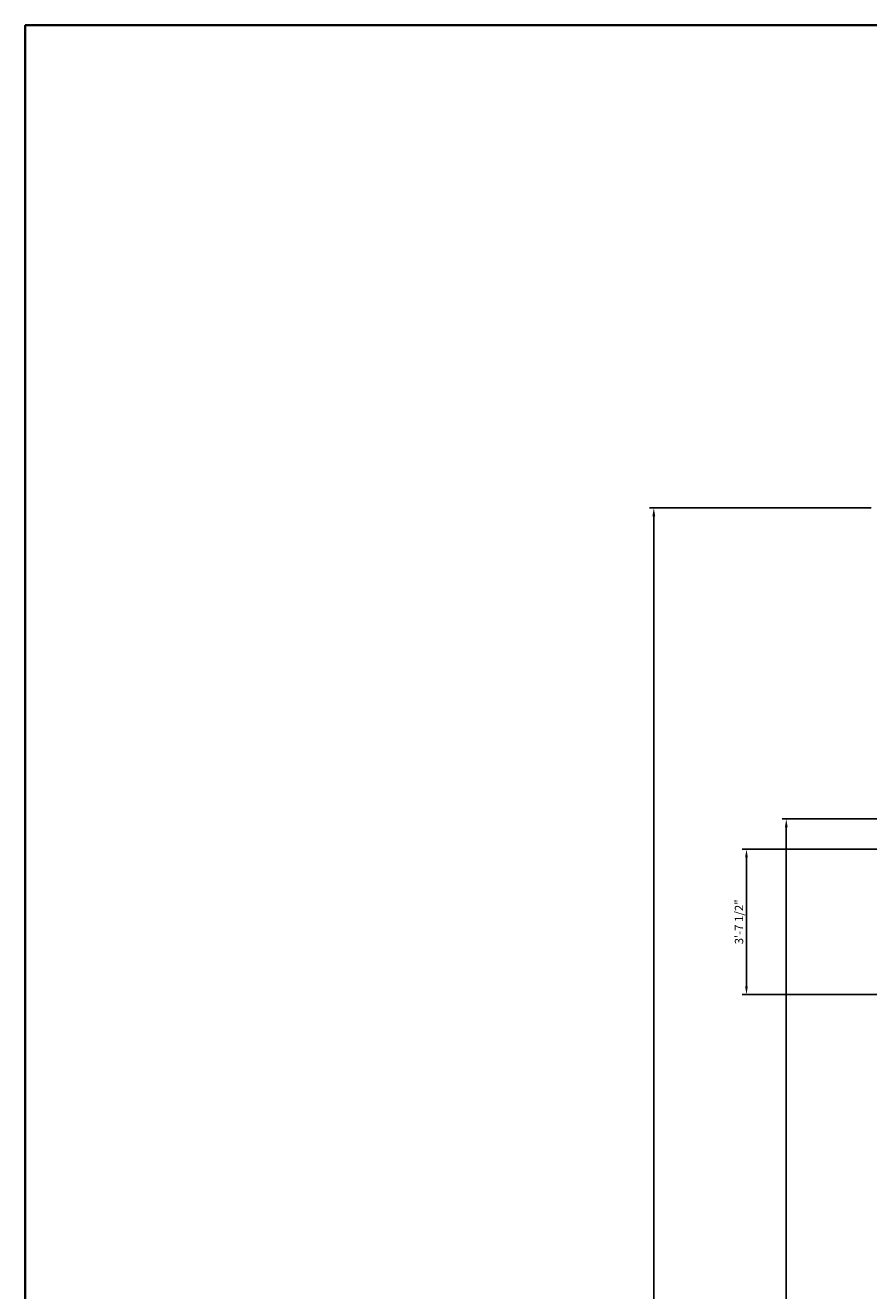
# Model space of a CAD drawing. Units: inches. Extents: x 6038 to 7543, y 3772 to 5131.
# Tile 7 of 14: x 6038 to 6290, y 4753 to 5131. Entities that reach past the tile are written whole.
import ezdxf

# ---------------------------------------------------------------- set-up
doc = ezdxf.new("R2010")
doc.units = ezdxf.units.IN
doc.layers.add('A-ANNO-DIMS', color=4, linetype='Continuous', lineweight=18)
doc.layers.add('A-ANNO-TTLB', color=1, linetype='Continuous', lineweight=35)
doc.styles.get("Standard").update_dxf_attribs({"font": 'arial.ttf'})
doc.dimstyles.new('ISO-25', dxfattribs={"dimtxt": 2.5, "dimasz": 2.5, "dimexe": 1.25, "dimexo": 0.625, "dimtad": 1, "dimdec": 0, "dimlunit": 3, "dimtxsty": 'Standard', "dimcen": 2.5, "dimadec": 0, "dimazin": 0, "dimtfac": 1, "dimtdec": 0, "dimtmove": 0, "dimatfit": 3, "dimfxl": 1, "dimarcsym": 0})

# ---------------------------------------------------------------- blocks, each defined once
blk = doc.blocks.new('*D15')
at = {"layer": 'A-ANNO-DIMS', "color": 0, "lineweight": -2, "transparency": 16777216}
for p, q in [((6320.79, 4893.62), (6264.12, 4893.62)), ((6265.37, 4891.12), (6265.37, 4551.12)), ((6320.79, 4548.62), (6264.12, 4548.62))]:
    blk.add_line(p, q, dxfattribs=at)
at = {"layer": 'A-ANNO-DIMS', "color": 0, "transparency": 16777216}
for points in [[(6264.96, 4891.12), (6265.79, 4891.12), (6265.37, 4893.62)], [(6264.96, 4551.12), (6265.79, 4551.12), (6265.37, 4548.62)]]:
    blk.add_solid(points, dxfattribs=at)
at = {"layer": 'Defpoints', "color": 0, "transparency": 16777216}
for p in [(6321.42, 4893.62), (6265.37, 4548.62), (6321.42, 4548.62)]:
    blk.add_point(p, dxfattribs=at)
at = {"layer": 'A-ANNO-DIMS', "color": 0, "transparency": 16777216, "insert": (6257.09, 4721.12), "char_height": 2.5, "attachment_point": 5, "rotation": 90}
blk.add_mtext('{\\H6x;28\'-9"}', dxfattribs=at)
blk = doc.blocks.new('*D17')
at = {"layer": 'A-ANNO-DIMS', "color": 0, "lineweight": -2, "transparency": 16777216}
for p, q in [((6290.79, 4986.62), (6224.51, 4986.62)), ((6225.76, 4984.12), (6225.76, 4365.12)), ((6290.79, 4362.62), (6224.51, 4362.62))]:
    blk.add_line(p, q, dxfattribs=at)
at = {"layer": 'A-ANNO-DIMS', "color": 0, "transparency": 16777216}
for points in [[(6225.34, 4984.12), (6226.18, 4984.12), (6225.76, 4986.62)], [(6225.34, 4365.12), (6226.18, 4365.12), (6225.76, 4362.62)]]:
    blk.add_solid(points, dxfattribs=at)
at = {"layer": 'Defpoints', "color": 0, "transparency": 16777216}
for p in [(6291.42, 4986.62), (6225.76, 4362.62), (6291.42, 4362.62)]:
    blk.add_point(p, dxfattribs=at)
at = {"layer": 'A-ANNO-DIMS', "color": 0, "transparency": 16777216, "insert": (6216.45, 4674.62), "char_height": 2.5, "attachment_point": 5, "rotation": 90}
blk.add_mtext("{\\H6.8x;52'}", dxfattribs=at)
blk = doc.blocks.new('*D62')
at = {"layer": 'A-ANNO-DIMS', "color": 0, "lineweight": -2, "transparency": 16777216}
for p, q in [((6329.79, 4884.62), (6252.22, 4884.62)), ((6253.47, 4843.62), (6253.47, 4882.12)), ((6329.79, 4841.12), (6252.22, 4841.12))]:
    blk.add_line(p, q, dxfattribs=at)
at = {"layer": 'A-ANNO-DIMS', "color": 0, "transparency": 16777216}
for points in [[(6253.05, 4882.12), (6253.88, 4882.12), (6253.47, 4884.62)], [(6253.05, 4843.62), (6253.88, 4843.62), (6253.47, 4841.12)]]:
    blk.add_solid(points, dxfattribs=at)
at = {"layer": 'Defpoints', "color": 0, "transparency": 16777216}
for p in [(6253.47, 4884.62), (6330.42, 4884.62), (6330.42, 4841.12)]:
    blk.add_point(p, dxfattribs=at)
at = {"layer": 'A-ANNO-DIMS', "color": 0, "transparency": 16777216, "insert": (6251.55, 4862.87), "char_height": 2.5, "attachment_point": 5, "rotation": 90}
blk.add_mtext('3\'-7 1/2"', dxfattribs=at)

msp = doc.modelspace()

# ---------------------------------------------------------------- linework, layer by layer
at = {"layer": 'A-ANNO-TTLB'}
msp.add_lwpolyline([(6037.83, 5130.86), (7542.53, 5130.86), (7542.53, 3772.09), (6037.83, 3772.09)], close=True, dxfattribs=at)

# ---------------------------------------------------------------- dimensions: what is measured, and where the dimension line sits
at = {"layer": 'A-ANNO-DIMS'}
dim = msp.add_linear_dim(base=(6225.76, 4362.62), p1=(6291.42, 4986.62), p2=(6291.42, 4362.62), angle=90, text='{\\H6.8x;<>}', dimstyle='ISO-25', override={"dimclrd": 0, "dimclre": 0, "dimclrt": 0}, dxfattribs=at)
dim.commit()
dim.dimension.update_dxf_attribs({"geometry": '*D17', "text_midpoint": (6225.76, 4674.62), "dimtype": 160})
dim = msp.add_linear_dim(base=(6265.37, 4548.62), p1=(6321.42, 4893.62), p2=(6321.42, 4548.62), angle=90, text='{\\H6x;<>}', dimstyle='ISO-25', override={"dimclrd": 0, "dimclre": 0, "dimclrt": 0}, dxfattribs=at)
dim.commit()
dim.dimension.update_dxf_attribs({"geometry": '*D15', "text_midpoint": (6257.09, 4721.12)})
dim = msp.add_linear_dim(base=(6253.47, 4884.62), p1=(6330.42, 4841.12), p2=(6330.42, 4884.62), angle=90, dimstyle='ISO-25', override={"dimdec": 1, "dimlfac": 1, "dimrnd": 0, "dimzin": 1, "dimdsep": 46, "dimlunit": 4, "dimfrac": 2}, dxfattribs=at)
dim.commit()
dim.dimension.update_dxf_attribs({"geometry": '*D62', "text_midpoint": (6251.55, 4862.87)})

doc.saveas('drawing.dxf')
